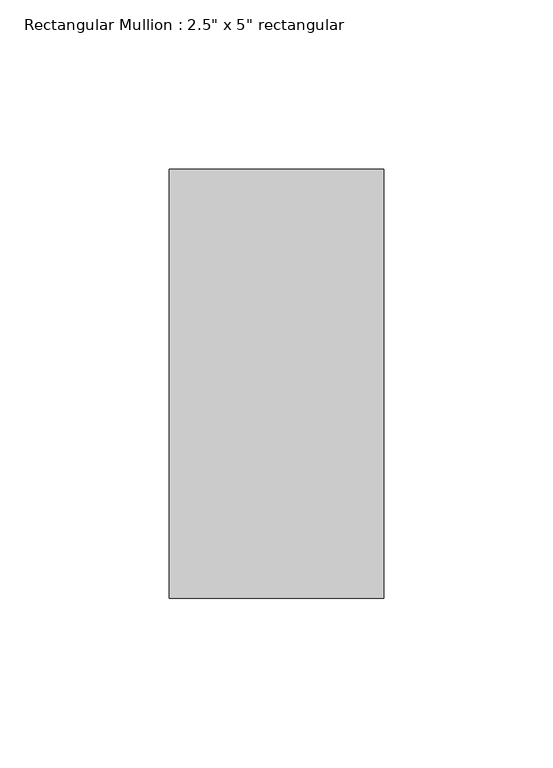
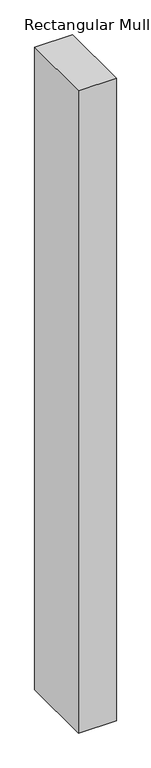
"""IFC4 building model written with IfcOpenShell, lengths in millimetres: member geometry."""

from ifc_helpers import new_model, si_unit, frame, origin, place, context, project, spatial, polyline, outline, extrude, source, transform, mapped, element, save


def member_7034f759(model_context):
    return source(origin(), model_context, "Body", "SweptSolid", [
        extrude(outline(polyline([(31.75, 63.5), (31.75, -63.5), (-31.75, -63.5), (-31.75, 63.5), (31.75, 63.5)])), frame((0.0, 0.0, -1137.9026335), z_axis=(0.0, 0.0, 1.0), x_axis=(1.0, 0.0, 0.0)), (0.0, 0.0, 1.0), 1137.9026335),
    ])


if __name__ == "__main__":
    model = new_model("IFC4")
    model_context = context("Model", 3, world=origin())
    ifc_project = project(units=[si_unit("LENGTHUNIT", "METRE", prefix="MILLI")], contexts=[model_context])
    site = spatial("IfcSite", under=ifc_project)
    building = spatial("IfcBuilding", under=site)
    placement = place(None, origin())
    member_shape = member_7034f759(model_context)
    element("IfcMember", 1, ObjectType="Rectangular Mullion : 2.5\" x 5\" rectangular", at=placement, inside=building, context=model_context, shape_type="MappedRepresentation", body=[
        mapped(member_shape, transform((0.0, 0.0, 0.0), x_axis=(1.0, 0.0, 0.0), y_axis=(0.0, 1.0, 0.0), z_axis=(0.0, 0.0, 1.0))),
    ])
    save(model, "model.ifc")

# Revit data of these elements
# Type "Rectangular Mullion : 2.5\" x 5\" rectangular"
#   built-in parameter 1007304 = 0.416667 (stored number, unit not read)
#   built-in parameter 1007301 = 0.104167 (stored number, unit not read)
#   built-in parameter 1007300 = 0.104167 (stored number, unit not read)
# Element 1 (IfcMember, "Rectangular Mullion : 2.5\" x 5\" rectangular")
#   Materials on its faces: "Aluminum"
# Materials
#   "Aluminum": class "Metal", colour RGB 247 247 247, transparency 0, Description = "Aluminum 6061", Cost = 0
